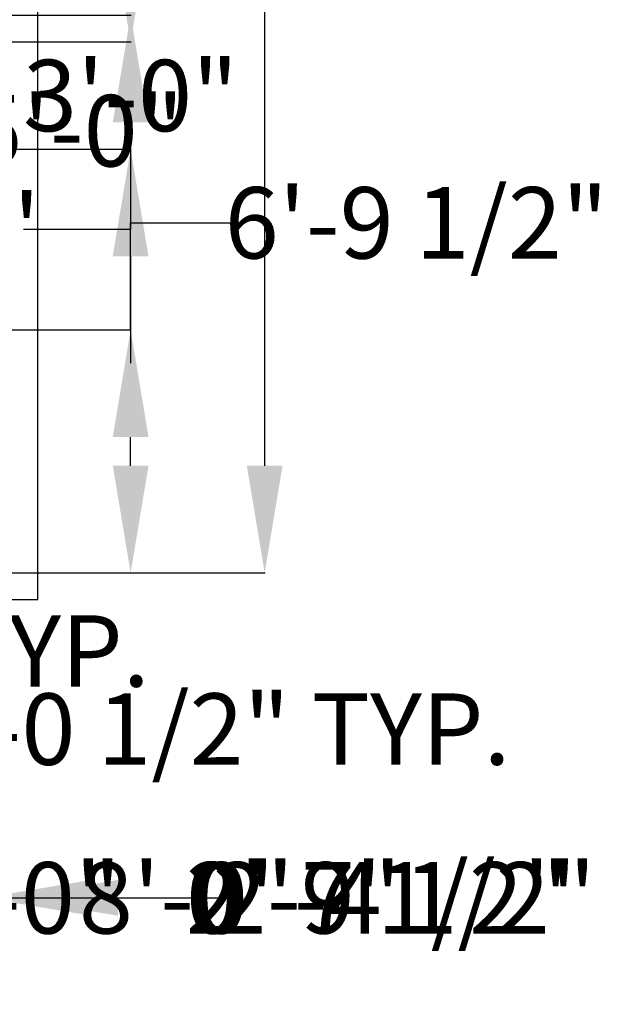
# Model space of a CAD drawing. Units: inches. Extents: x 2838 to 4029, y 1041 to 1915.
# Tile 4 of 16: x 3631 to 3825, y 1046 to 1377. Entities that reach past the tile are written whole.
import ezdxf

# ---------------------------------------------------------------- set-up
doc = ezdxf.new("R2010")
doc.units = ezdxf.units.IN
doc.header["$MEASUREMENT"] = 0
doc.layers.add('A-ANNO-DIMS', color=2, linetype='Continuous', lineweight=18)
doc.layers.add('A-FLOR', color=7, linetype='Continuous', lineweight=25)
doc.styles.get("Standard").update_dxf_attribs({"font": 'arial.ttf'})
doc.dimstyles.get("Standard").update_dxf_attribs({"dimtxt": 24, "dimasz": 36, "dimexe": 0.18, "dimexo": 0.0625, "dimgap": 0.09, "dimtad": 0, "dimtih": 1, "dimtoh": 1, "dimdec": 0, "dimzin": 0, "dimdsep": 46, "dimlunit": 3, "dimtxsty": 'Standard', "dimcen": 0.09, "dimadec": 0, "dimazin": 0, "dimtfac": 1, "dimtdec": 0, "dimtofl": 0, "dimtmove": 0, "dimatfit": 3, "dimfxl": 1, "dimtolj": 1, "dimtzin": 0, "dimarcsym": 0})

# ---------------------------------------------------------------- blocks, each defined once
blk = doc.blocks.new('*D17')
at = {"layer": 'A-ANNO-DIMS', "color": 0, "lineweight": -2, "transparency": 16777216}
for p, q in [((3627.79, 1671.3), (3713.18, 1671.3)), ((3713, 1635.3), (3713, 1443.64)), ((3713, 1227.3), (3713, 1418.95)), ((3627.79, 1191.3), (3713.18, 1191.3))]:
    blk.add_line(p, q, dxfattribs=at)
at = {"layer": 'A-ANNO-DIMS', "color": 0, "transparency": 16777216}
for points in [[(3707, 1635.3), (3719, 1635.3), (3713, 1671.3)], [(3707, 1227.3), (3719, 1227.3), (3713, 1191.3)]]:
    blk.add_solid(points, dxfattribs=at)
at = {"layer": 'Defpoints', "color": 0, "transparency": 16777216}
for p in [(3627.73, 1671.3), (3627.73, 1191.3), (3713, 1191.3)]:
    blk.add_point(p, dxfattribs=at)
at = {"layer": 'A-ANNO-DIMS', "color": 0, "transparency": 16777216, "insert": (3713, 1431.3), "char_height": 24, "attachment_point": 5}
blk.add_mtext("\\A1;40'", dxfattribs=at)
blk = doc.blocks.new('*D29')
at = {"layer": 'A-ANNO-DIMS', "color": 0, "lineweight": -2, "transparency": 16777216}
for p, q in [((3310.15, 1348.85), (3310.15, 1339.73)), ((3370.15, 1348.85), (3370.15, 1339.73)), ((3274.15, 1339.91), (3238.15, 1339.91)), ((3406.15, 1339.91), (3442.15, 1339.91))]:
    blk.add_line(p, q, dxfattribs=at)
at = {"layer": 'A-ANNO-DIMS', "color": 0, "transparency": 16777216}
for points in [[(3274.15, 1345.91), (3274.15, 1333.91), (3310.15, 1339.91)], [(3406.15, 1345.91), (3406.15, 1333.91), (3370.15, 1339.91)]]:
    blk.add_solid(points, dxfattribs=at)
at = {"layer": 'Defpoints', "color": 0, "transparency": 16777216}
for p in [(3310.15, 1348.91), (3370.15, 1348.91), (3370.15, 1339.91)]:
    blk.add_point(p, dxfattribs=at)
at = {"layer": 'A-ANNO-DIMS', "color": 0, "transparency": 16777216, "insert": (3566.77, 1339.91), "char_height": 24, "attachment_point": 5}
blk.add_mtext('\\A1;LOVESEAT 5\'-0"', dxfattribs=at)
blk = doc.blocks.new('*D31')
at = {"layer": 'A-ANNO-DIMS', "color": 0, "lineweight": -2, "transparency": 16777216}
for p, q in [((3489.98, 1221.23), (3489.98, 1257.23)), ((3495.97, 1185.23), (3489.8, 1185.23)), ((3495.97, 1144.84), (3489.8, 1144.84)), ((3489.98, 1108.84), (3489.98, 1072.84))]:
    blk.add_line(p, q, dxfattribs=at)
at = {"layer": 'A-ANNO-DIMS', "color": 0, "transparency": 16777216}
for points in [[(3483.98, 1221.23), (3495.98, 1221.23), (3489.98, 1185.23)], [(3483.98, 1108.84), (3495.98, 1108.84), (3489.98, 1144.84)]]:
    blk.add_solid(points, dxfattribs=at)
at = {"layer": 'Defpoints', "color": 0, "transparency": 16777216}
for p in [(3496.03, 1185.23), (3489.98, 1144.84), (3496.03, 1144.84)]:
    blk.add_point(p, dxfattribs=at)
at = {"layer": 'A-ANNO-DIMS', "color": 0, "transparency": 16777216, "insert": (3489.98, 1165.04), "char_height": 24, "attachment_point": 5}
blk.add_mtext('\\A1;LOVESEAT 3\'-4 1/2" TYP.', dxfattribs=at)
blk = doc.blocks.new('*D32')
at = {"layer": 'A-ANNO-DIMS', "color": 0, "lineweight": -2, "transparency": 16777216}
for p, q in [((3496.03, 1144.78), (3496.03, 1138.61)), ((3520.71, 1144.78), (3520.71, 1138.61)), ((3460.03, 1138.79), (3424.03, 1138.79)), ((3556.71, 1138.79), (3592.71, 1138.79))]:
    blk.add_line(p, q, dxfattribs=at)
at = {"layer": 'A-ANNO-DIMS', "color": 0, "transparency": 16777216}
for points in [[(3460.03, 1144.79), (3460.03, 1132.79), (3496.03, 1138.79)], [(3556.71, 1144.79), (3556.71, 1132.79), (3520.71, 1138.79)]]:
    blk.add_solid(points, dxfattribs=at)
at = {"layer": 'Defpoints', "color": 0, "transparency": 16777216}
for p in [(3496.03, 1144.84), (3520.71, 1144.84), (3520.71, 1138.79)]:
    blk.add_point(p, dxfattribs=at)
at = {"layer": 'A-ANNO-DIMS', "color": 0, "transparency": 16777216, "insert": (3694.12, 1138.79), "char_height": 24, "attachment_point": 5}
blk.add_mtext('\\A1;2\'-0 1/2" TYP.', dxfattribs=at)
blk = doc.blocks.new('*D49')
at = {"layer": 'A-ANNO-DIMS', "color": 0, "lineweight": -2, "transparency": 16777216}
for p, q in [((3336.37, 1426.68), (3336.37, 1412.92)), ((3427.37, 1426.68), (3427.37, 1412.92)), ((3372.37, 1413.1), (3391.37, 1413.1)), ((3427.37, 1413.1), (3463.37, 1413.1))]:
    blk.add_line(p, q, dxfattribs=at)
at = {"layer": 'A-ANNO-DIMS', "color": 0, "transparency": 16777216}
for points in [[(3372.37, 1419.1), (3372.37, 1407.1), (3336.37, 1413.1)], [(3391.37, 1419.1), (3391.37, 1407.1), (3427.37, 1413.1)]]:
    blk.add_solid(points, dxfattribs=at)
at = {"layer": 'Defpoints', "color": 0, "transparency": 16777216}
for p in [(3336.37, 1426.75), (3427.37, 1426.75), (3427.37, 1413.1)]:
    blk.add_point(p, dxfattribs=at)
at = {"layer": 'A-ANNO-DIMS', "color": 0, "transparency": 16777216, "insert": (3595.36, 1413.1), "char_height": 24, "attachment_point": 5}
blk.add_mtext('\\A1;DINING SET 7\'-7"', dxfattribs=at)
blk = doc.blocks.new('*D53')
at = {"layer": 'A-ANNO-DIMS', "color": 0, "lineweight": -2, "transparency": 16777216}
for p, q in [((3583.96, 1508.36), (3583.96, 1544.36)), ((3588.4, 1472.36), (3583.78, 1472.36)), ((3588.4, 1442.36), (3583.78, 1442.36)), ((3583.96, 1406.36), (3583.96, 1370.36))]:
    blk.add_line(p, q, dxfattribs=at)
at = {"layer": 'A-ANNO-DIMS', "color": 0, "transparency": 16777216}
for points in [[(3577.96, 1508.36), (3589.96, 1508.36), (3583.96, 1472.36)], [(3577.96, 1406.36), (3589.96, 1406.36), (3583.96, 1442.36)]]:
    blk.add_solid(points, dxfattribs=at)
at = {"layer": 'Defpoints', "color": 0, "transparency": 16777216}
for p in [(3588.46, 1472.36), (3583.96, 1442.36), (3588.46, 1442.36)]:
    blk.add_point(p, dxfattribs=at)
at = {"layer": 'A-ANNO-DIMS', "color": 0, "transparency": 16777216, "insert": (3583.96, 1457.36), "char_height": 24, "attachment_point": 5}
blk.add_mtext('\\A1;RANGE 2\'-6"', dxfattribs=at)
blk = doc.blocks.new('*D57')
at = {"layer": 'A-ANNO-DIMS', "color": 0, "lineweight": -2, "transparency": 16777216}
for p, q in [((3585.57, 1472.38), (3585.57, 1508.38)), ((3590.9, 1436.38), (3585.39, 1436.38)), ((3590.9, 1400.38), (3585.39, 1400.38)), ((3585.57, 1364.38), (3585.57, 1328.38))]:
    blk.add_line(p, q, dxfattribs=at)
at = {"layer": 'A-ANNO-DIMS', "color": 0, "transparency": 16777216}
for points in [[(3579.57, 1472.38), (3591.57, 1472.38), (3585.57, 1436.38)], [(3579.57, 1364.38), (3591.57, 1364.38), (3585.57, 1400.38)]]:
    blk.add_solid(points, dxfattribs=at)
at = {"layer": 'Defpoints', "color": 0, "transparency": 16777216}
for p in [(3590.97, 1436.38), (3585.57, 1400.38), (3590.97, 1400.38)]:
    blk.add_point(p, dxfattribs=at)
at = {"layer": 'A-ANNO-DIMS', "color": 0, "transparency": 16777216, "insert": (3585.57, 1418.38), "char_height": 24, "attachment_point": 5}
blk.add_mtext('\\A1;DOUBLE SINK 3\'-0"', dxfattribs=at)
blk = doc.blocks.new('*D73')
at = {"layer": 'A-ANNO-DIMS', "color": 0, "lineweight": -2, "transparency": 16777216}
for p, q in [((3425.038746, 1711.522346), (3389.038746, 1711.522346)), ((3461.038746, 1200.359846), (3461.038746, 1711.702346)), ((3618.731626, 1200.359846), (3618.731626, 1711.702346)), ((3654.731626, 1711.522346), (3690.731626, 1711.522346))]:
    blk.add_line(p, q, dxfattribs=at)
at = {"layer": 'A-ANNO-DIMS', "color": 0, "transparency": 16777216}
for points in [[(3425.038746, 1717.522346), (3425.038746, 1705.522346), (3461.038746, 1711.522346)], [(3654.731626, 1717.522346), (3654.731626, 1705.522346), (3618.731626, 1711.522346)]]:
    blk.add_solid(points, dxfattribs=at)
at = {"layer": 'Defpoints', "color": 0, "transparency": 16777216}
for p in [(3618.731626, 1711.522346), (3461.038746, 1200.297346), (3618.731626, 1200.297346)]:
    blk.add_point(p, dxfattribs=at)
at = {"layer": 'A-ANNO-DIMS', "color": 0, "transparency": 16777216, "insert": (3539.885186, 1711.522346), "char_height": 24, "attachment_point": 5}
blk.add_mtext('\\A1;13\'-1 1/2"', dxfattribs=at)
blk = doc.blocks.new('*D74')
at = {"layer": 'A-ANNO-DIMS', "color": 0, "lineweight": -2, "transparency": 16777216}
for p, q in [((3513.73, 1297.66), (3513.73, 1081.89)), ((3525.73, 1297.66), (3525.73, 1081.89)), ((3477.73, 1082.07), (3441.73, 1082.07)), ((3561.73, 1082.07), (3597.73, 1082.07))]:
    blk.add_line(p, q, dxfattribs=at)
at = {"layer": 'A-ANNO-DIMS', "color": 0, "transparency": 16777216}
for points in [[(3477.73, 1088.07), (3477.73, 1076.07), (3513.73, 1082.07)], [(3561.73, 1088.07), (3561.73, 1076.07), (3525.73, 1082.07)]]:
    blk.add_solid(points, dxfattribs=at)
at = {"layer": 'Defpoints', "color": 0, "transparency": 16777216}
for p in [(3513.73, 1297.73), (3525.73, 1297.73), (3525.73, 1082.07)]:
    blk.add_point(p, dxfattribs=at)
at = {"layer": 'A-ANNO-DIMS', "color": 0, "transparency": 16777216, "insert": (3628.59, 1082.07), "char_height": 24, "attachment_point": 5}
blk.add_mtext('\\A1;1\'-0"', dxfattribs=at)
blk = doc.blocks.new('*D75')
at = {"layer": 'A-ANNO-DIMS', "color": 0, "lineweight": -2, "transparency": 16777216}
for p, q in [((3667.956626, 1405.727214), (3667.956626, 1441.727214)), ((3618.794126, 1369.727214), (3668.136626, 1369.727214)), ((3618.794126, 1333.727214), (3668.136626, 1333.727214)), ((3667.956626, 1297.727214), (3667.956626, 1261.727214))]:
    blk.add_line(p, q, dxfattribs=at)
at = {"layer": 'A-ANNO-DIMS', "color": 0, "transparency": 16777216}
for points in [[(3661.956626, 1405.727214), (3673.956626, 1405.727214), (3667.956626, 1369.727214)], [(3661.956626, 1297.727214), (3673.956626, 1297.727214), (3667.956626, 1333.727214)]]:
    blk.add_solid(points, dxfattribs=at)
at = {"layer": 'Defpoints', "color": 0, "transparency": 16777216}
for p in [(3618.731626, 1369.727214), (3667.956626, 1369.727214), (3618.731626, 1333.727214)]:
    blk.add_point(p, dxfattribs=at)
at = {"layer": 'A-ANNO-DIMS', "color": 0, "transparency": 16777216, "insert": (3667.956626, 1351.727214), "char_height": 24, "attachment_point": 5}
blk.add_mtext('\\A1;3\'-0"', dxfattribs=at)
blk = doc.blocks.new('*D88')
at = {"layer": 'A-ANNO-DIMS', "color": 0, "lineweight": -2, "transparency": 16777216}
for p, q in [((3522.73, 1378.66), (3522.73, 1081.89)), ((3618.73, 1378.66), (3618.73, 1081.89)), ((3558.73, 1082.07), (3582.73, 1082.07)), ((3618.73, 1082.07), (3654.73, 1082.07))]:
    blk.add_line(p, q, dxfattribs=at)
at = {"layer": 'A-ANNO-DIMS', "color": 0, "transparency": 16777216}
for points in [[(3558.73, 1088.07), (3558.73, 1076.07), (3522.73, 1082.07)], [(3582.73, 1088.07), (3582.73, 1076.07), (3618.73, 1082.07)]]:
    blk.add_solid(points, dxfattribs=at)
at = {"layer": 'Defpoints', "color": 0, "transparency": 16777216}
for p in [(3522.73, 1378.73), (3618.73, 1378.73), (3618.73, 1082.07)]:
    blk.add_point(p, dxfattribs=at)
at = {"layer": 'A-ANNO-DIMS', "color": 0, "transparency": 16777216, "insert": (3686.74, 1082.07), "char_height": 24, "attachment_point": 5}
blk.add_mtext('\\A1;8\'-0"', dxfattribs=at)
blk = doc.blocks.new('*D90')
at = {"layer": 'A-ANNO-DIMS', "color": 0, "lineweight": -2, "transparency": 16777216}
for p, q in [((3667.96, 1457.85), (3667.96, 1493.85)), ((3618.79, 1421.85), (3668.14, 1421.85)), ((3618.79, 1378.73), (3668.14, 1378.73)), ((3667.96, 1342.73), (3667.96, 1306.73))]:
    blk.add_line(p, q, dxfattribs=at)
at = {"layer": 'A-ANNO-DIMS', "color": 0, "transparency": 16777216}
for points in [[(3661.96, 1457.85), (3673.96, 1457.85), (3667.96, 1421.85)], [(3661.96, 1342.73), (3673.96, 1342.73), (3667.96, 1378.73)]]:
    blk.add_solid(points, dxfattribs=at)
at = {"layer": 'Defpoints', "color": 0, "transparency": 16777216}
for p in [(3618.73, 1421.85), (3667.96, 1421.85), (3618.73, 1378.73)]:
    blk.add_point(p, dxfattribs=at)
at = {"layer": 'A-ANNO-DIMS', "color": 0, "transparency": 16777216, "insert": (3667.96, 1400.29), "char_height": 24, "attachment_point": 5}
blk.add_mtext('\\A1;3\'-7"', dxfattribs=at)
blk = doc.blocks.new('*D92')
at = {"layer": 'A-ANNO-DIMS', "color": 0, "lineweight": -2, "transparency": 16777216}
for p, q in [((3585.37, 1402), (3585.37, 1081.89)), ((3618.73, 1378.66), (3618.73, 1081.89)), ((3549.37, 1082.07), (3513.37, 1082.07)), ((3654.73, 1082.07), (3690.73, 1082.07))]:
    blk.add_line(p, q, dxfattribs=at)
at = {"layer": 'A-ANNO-DIMS', "color": 0, "transparency": 16777216}
for points in [[(3549.37, 1088.07), (3549.37, 1076.07), (3585.37, 1082.07)], [(3654.73, 1088.07), (3654.73, 1076.07), (3618.73, 1082.07)]]:
    blk.add_solid(points, dxfattribs=at)
at = {"layer": 'Defpoints', "color": 0, "transparency": 16777216}
for p in [(3585.37, 1402.06), (3618.73, 1378.73), (3618.73, 1082.07)]:
    blk.add_point(p, dxfattribs=at)
at = {"layer": 'A-ANNO-DIMS', "color": 0, "transparency": 16777216, "insert": (3750.89, 1082.07), "char_height": 24, "attachment_point": 5}
blk.add_mtext('\\A1;2\'-9 1/2"', dxfattribs=at)
blk = doc.blocks.new('*D98')
at = {"layer": 'A-ANNO-DIMS', "color": 0, "lineweight": -2, "transparency": 16777216}
for p, q in [((3667.96, 1272.94), (3667.96, 1308.94)), ((3667.96, 1308.94), (3703.96, 1308.94)), ((3627.79, 1272.94), (3668.14, 1272.94)), ((3667.96, 1227.3), (3667.96, 1236.94)), ((3627.79, 1191.3), (3668.14, 1191.3))]:
    blk.add_line(p, q, dxfattribs=at)
at = {"layer": 'A-ANNO-DIMS', "color": 0, "transparency": 16777216}
for points in [[(3661.96, 1236.94), (3673.96, 1236.94), (3667.96, 1272.94)], [(3661.96, 1227.3), (3673.96, 1227.3), (3667.96, 1191.3)]]:
    blk.add_solid(points, dxfattribs=at)
at = {"layer": 'Defpoints', "color": 0, "transparency": 16777216}
for p in [(3627.73, 1272.94), (3667.96, 1272.94), (3627.73, 1191.3)]:
    blk.add_point(p, dxfattribs=at)
at = {"layer": 'A-ANNO-DIMS', "color": 0, "transparency": 16777216, "insert": (3763.97, 1308.94), "char_height": 24, "attachment_point": 5}
blk.add_mtext('\\A1;6\'-9 1/2"', dxfattribs=at)
blk = doc.blocks.new('*D99')
at = {"layer": 'A-ANNO-DIMS', "color": 0, "lineweight": -2, "transparency": 16777216}
for p, q in [((3599.07, 1191.23), (3599.07, 1081.89)), ((3627.73, 1191.23), (3627.73, 1081.89)), ((3563.07, 1082.07), (3527.07, 1082.07)), ((3663.73, 1082.07), (3699.73, 1082.07))]:
    blk.add_line(p, q, dxfattribs=at)
at = {"layer": 'A-ANNO-DIMS', "color": 0, "transparency": 16777216}
for points in [[(3563.07, 1088.07), (3563.07, 1076.07), (3599.07, 1082.07)], [(3663.73, 1088.07), (3663.73, 1076.07), (3627.73, 1082.07)]]:
    blk.add_solid(points, dxfattribs=at)
at = {"layer": 'Defpoints', "color": 0, "transparency": 16777216}
for p in [(3599.07, 1191.3), (3627.73, 1191.3), (3627.73, 1082.07)]:
    blk.add_point(p, dxfattribs=at)
at = {"layer": 'A-ANNO-DIMS', "color": 0, "transparency": 16777216, "insert": (3759.89, 1082.07), "char_height": 24, "attachment_point": 5}
blk.add_mtext('\\A1;2\'-4 1/2"', dxfattribs=at)
blk = doc.blocks.new('*D106')
at = {"layer": 'A-ANNO-DIMS', "color": 0, "lineweight": -2, "transparency": 16777216}
for p, q in [((3611.97, 1401.82), (3611.97, 1081.89)), ((3618.73, 1378.66), (3618.73, 1081.89)), ((3575.97, 1082.07), (3539.97, 1082.07)), ((3654.73, 1082.07), (3690.73, 1082.07))]:
    blk.add_line(p, q, dxfattribs=at)
at = {"layer": 'A-ANNO-DIMS', "color": 0, "transparency": 16777216}
for points in [[(3575.97, 1088.07), (3575.97, 1076.07), (3611.97, 1082.07)], [(3654.73, 1088.07), (3654.73, 1076.07), (3618.73, 1082.07)]]:
    blk.add_solid(points, dxfattribs=at)
at = {"layer": 'Defpoints', "color": 0, "transparency": 16777216}
for p in [(3611.97, 1401.88), (3618.73, 1378.73), (3618.73, 1082.07)]:
    blk.add_point(p, dxfattribs=at)
at = {"layer": 'A-ANNO-DIMS', "color": 0, "transparency": 16777216, "insert": (3722.72, 1082.07), "char_height": 24, "attachment_point": 5}
blk.add_mtext('\\A1;0\'-7"', dxfattribs=at)
blk = doc.blocks.new('*D107')
at = {"layer": 'A-ANNO-DIMS', "color": 0, "lineweight": -2, "transparency": 16777216}
for p, q in [((3667.96, 1436.38), (3667.96, 1472.38)), ((3610.53, 1400.38), (3668.14, 1400.38)), ((3618.79, 1378.73), (3668.14, 1378.73)), ((3667.96, 1342.73), (3667.96, 1306.73)), ((3667.96, 1306.73), (3631.96, 1306.73))]:
    blk.add_line(p, q, dxfattribs=at)
at = {"layer": 'A-ANNO-DIMS', "color": 0, "transparency": 16777216}
for points in [[(3661.96, 1436.38), (3673.96, 1436.38), (3667.96, 1400.38)], [(3661.96, 1342.73), (3673.96, 1342.73), (3667.96, 1378.73)]]:
    blk.add_solid(points, dxfattribs=at)
at = {"layer": 'Defpoints', "color": 0, "transparency": 16777216}
for p in [(3610.47, 1400.38), (3618.73, 1378.73), (3667.96, 1378.73)]:
    blk.add_point(p, dxfattribs=at)
at = {"layer": 'A-ANNO-DIMS', "color": 0, "transparency": 16777216, "insert": (3573.14, 1306.73), "char_height": 24, "attachment_point": 5}
blk.add_mtext('\\A1;1\'-9 1/2"', dxfattribs=at)

msp = doc.modelspace()

# ---------------------------------------------------------------- linework, layer by layer
at = {"layer": 'A-FLOR'}
msp.add_lwpolyline([(3527.95, 1182.3), (3636.73, 1182.3), (3636.73, 1680.3), (3258.73, 1680.3), (3258.73, 1182.3), (3267.73, 1182.3)], dxfattribs=at)

# ---------------------------------------------------------------- dimensions: what is measured, and where the dimension line sits
at = {"layer": 'A-ANNO-DIMS'}
for base, p1, p2, picture, middle in [((3618.73, 1711.52), (3461.04, 1200.3), (3618.73, 1200.3), '*D73', (3539.89, 1711.52)), ((3618.73, 1082.07), (3585.37, 1402.06), (3618.73, 1378.73), '*D92', (3750.89, 1082.07)), ((3618.73, 1082.07), (3611.97, 1401.88), (3618.73, 1378.73), '*D106', (3722.72, 1082.07)), ((3618.73, 1082.07), (3522.73, 1378.73), (3618.73, 1378.73), '*D88', (3686.74, 1082.07)), ((3525.73, 1082.07), (3513.73, 1297.73), (3525.73, 1297.73), '*D74', (3628.59, 1082.07)), ((3627.73, 1082.07), (3599.07, 1191.3), (3627.73, 1191.3), '*D99', (3759.89, 1082.07))]:
    dim = msp.add_linear_dim(base=base, p1=p1, p2=p2, dimstyle='Standard', override={"dimdec": 1, "dimlfac": 1, "dimrnd": 0, "dimzin": 1, "dimdsep": 46, "dimlunit": 4, "dimfrac": 2}, dxfattribs=at)
    dim.commit()
    dim.dimension.update_dxf_attribs({"geometry": picture, "text_midpoint": middle})
for base, p1, p2, override, picture, middle in [((3713, 1191.3), (3627.73, 1671.3), (3627.73, 1191.3), {"dimclrd": 0, "dimclre": 0, "dimclrt": 0}, '*D17', (3713, 1431.3)), ((3667.96, 1421.85), (3618.73, 1378.73), (3618.73, 1421.85), {"dimdec": 1, "dimlfac": 1, "dimrnd": 0, "dimzin": 1, "dimdsep": 46, "dimlunit": 4, "dimfrac": 2}, '*D90', (3667.96, 1400.29)), ((3667.9566, 1378.7272), (3610.4672, 1400.3841), (3618.7316, 1378.7272), {"dimdec": 1, "dimlfac": 1, "dimrnd": 0, "dimzin": 1, "dimdsep": 46, "dimlunit": 4, "dimfrac": 2}, '*D107', (3573.1354, 1306.7272)), ((3667.96, 1369.73), (3618.73, 1333.73), (3618.73, 1369.73), {"dimdec": 1, "dimlfac": 1, "dimrnd": 0, "dimzin": 1, "dimdsep": 46, "dimlunit": 4, "dimfrac": 2}, '*D75', (3667.96, 1351.73)), ((3667.96, 1272.94), (3627.73, 1191.3), (3627.73, 1272.94), {"dimdec": 1, "dimlfac": 1, "dimrnd": 0, "dimzin": 1, "dimdsep": 46, "dimlunit": 4, "dimfrac": 2}, '*D98', (3763.97, 1308.94))]:
    dim = msp.add_linear_dim(base=base, p1=p1, p2=p2, angle=90, dimstyle='Standard', override=override, dxfattribs=at)
    dim.commit()
    dim.dimension.update_dxf_attribs({"geometry": picture, "text_midpoint": middle})
for base, p1, p2, text, picture, middle in [((3583.96, 1442.36), (3588.46, 1472.36), (3588.46, 1442.36), 'RANGE <>', '*D53', (3583.96, 1457.36)), ((3585.57, 1400.38), (3590.97, 1436.38), (3590.97, 1400.38), 'DOUBLE SINK <>', '*D57', (3585.57, 1418.38)), ((3489.98, 1144.84), (3496.03, 1185.23), (3496.03, 1144.84), 'LOVESEAT <> TYP.', '*D31', (3489.98, 1165.04))]:
    dim = msp.add_linear_dim(base=base, p1=p1, p2=p2, angle=270, text=text, dimstyle='Standard', override={"dimdec": 1, "dimlfac": 1, "dimrnd": 0, "dimzin": 1, "dimdsep": 46, "dimlunit": 4, "dimfrac": 2}, dxfattribs=at)
    dim.commit()
    dim.dimension.update_dxf_attribs({"geometry": picture, "text_midpoint": middle})
for base, p1, p2, text, picture, middle in [((3427.37, 1413.1), (3336.37, 1426.75), (3427.37, 1426.75), 'DINING SET <>', '*D49', (3595.36, 1413.1)), ((3370.15, 1339.91), (3310.15, 1348.91), (3370.15, 1348.91), 'LOVESEAT <>', '*D29', (3566.77, 1339.91)), ((3520.71, 1138.79), (3496.03, 1144.84), (3520.71, 1144.84), '<> TYP.', '*D32', (3694.12, 1138.79))]:
    dim = msp.add_linear_dim(base=base, p1=p1, p2=p2, text=text, dimstyle='Standard', override={"dimdec": 1, "dimlfac": 1, "dimrnd": 0, "dimzin": 1, "dimdsep": 46, "dimlunit": 4, "dimfrac": 2}, dxfattribs=at)
    dim.commit()
    dim.dimension.update_dxf_attribs({"geometry": picture, "text_midpoint": middle})

doc.saveas('drawing.dxf')
